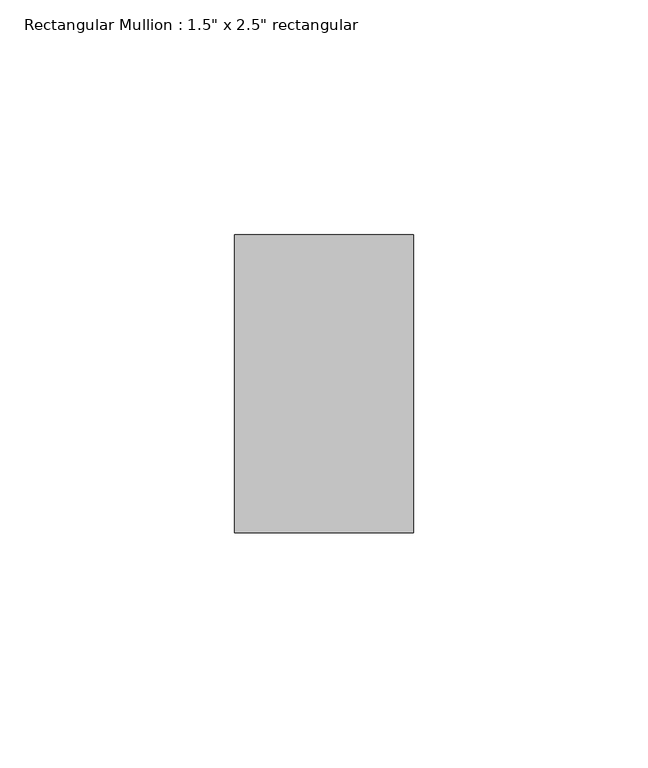
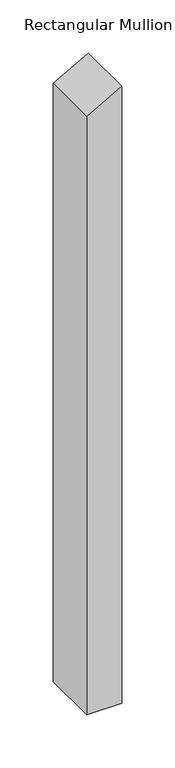
"""IFC4 building model written with IfcOpenShell, lengths in millimetres: member geometry."""

from ifc_helpers import new_model, si_unit, frame, origin, place, context, project, spatial, polyline, outline, extrude, source, transform, mapped, element, save


def member_06c20982(model_context):
    return source(origin(), model_context, "Body", "SweptSolid", [
        extrude(outline(polyline([(0.0, 0.0), (-21.676858, -38.1), (-710.2081316, -38.1), (-710.2081316, 0.0), (0.0, 0.0)])), frame((0.0, -31.75, 0.0), z_axis=(0.0, 1.0, 0.0), x_axis=(0.0, 0.0, 1.0)), (0.0, 0.0, 1.0), 63.5),
    ])


if __name__ == "__main__":
    model = new_model("IFC4")
    model_context = context("Model", 3, world=origin())
    ifc_project = project(units=[si_unit("LENGTHUNIT", "METRE", prefix="MILLI")], contexts=[model_context])
    site = spatial("IfcSite", under=ifc_project)
    building = spatial("IfcBuilding", under=site)
    placement = place(None, origin())
    member_shape = member_06c20982(model_context)
    element("IfcMember", 1, ObjectType="Rectangular Mullion : 1.5\" x 2.5\" rectangular", at=placement, inside=building, context=model_context, shape_type="MappedRepresentation", body=[
        mapped(member_shape, transform((0.0, 0.0, 0.0), x_axis=(1.0, 0.0, 0.0), y_axis=(0.0, 1.0, 0.0), z_axis=(0.0, 0.0, 1.0))),
    ])
    save(model, "model.ifc")

# Revit data of these elements
# Type "Rectangular Mullion : 1.5\" x 2.5\" rectangular"
#   built-in parameter 1007304 = 0.208333 (stored number, unit not read)
#   built-in parameter 1007301 = 0.0625 (stored number, unit not read)
#   built-in parameter 1007300 = 0.0625 (stored number, unit not read)
